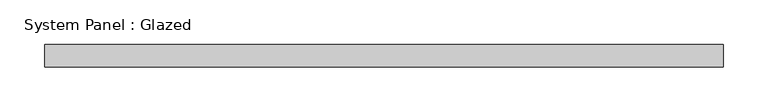
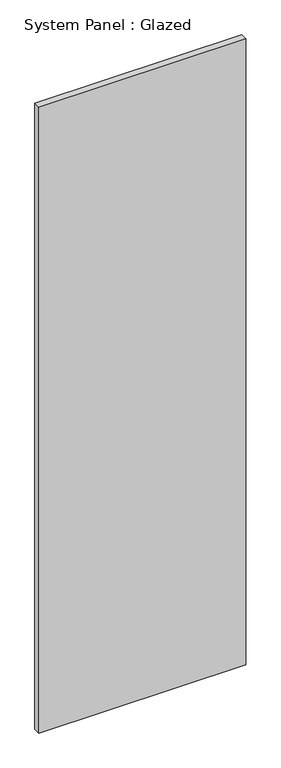
"""IFC4 building model written with IfcOpenShell, lengths in millimetres: plate geometry, System Panel : Glazed."""

from ifc_helpers import new_model, si_unit, origin, origin_with_axes, place, context, project, spatial, polyline, outline, extrude, source, transform, mapped, element, save


def system_panel_glazed_7cdb8ab2(model_context):
    return source(origin(), model_context, "Body", "SweptSolid", [
        extrude(outline(polyline([(381.0, 19.05), (-381.0, 19.05), (-381.0, 44.45), (381.0, 44.45), (381.0, 19.05)])), origin_with_axes(), (0.0, 0.0, 1.0), 2438.4),
    ])


if __name__ == "__main__":
    model = new_model("IFC4")
    model_context = context("Model", 3, world=origin())
    ifc_project = project(units=[si_unit("LENGTHUNIT", "METRE", prefix="MILLI")], contexts=[model_context])
    site = spatial("IfcSite", under=ifc_project)
    building = spatial("IfcBuilding", under=site)
    placement = place(None, origin())
    system_panel_glazed_shape = system_panel_glazed_7cdb8ab2(model_context)
    element("IfcPlate", 1, ObjectType="System Panel : Glazed", at=placement, inside=building, context=model_context, shape_type="MappedRepresentation", body=[
        mapped(system_panel_glazed_shape, transform((0.0, 0.0, 0.0), x_axis=(1.0, 0.0, 0.0), y_axis=(0.0, 1.0, 0.0), z_axis=(0.0, 0.0, 1.0))),
    ])
    save(model, "model.ifc")

# Revit data of these elements
# Type "System Panel : Glazed"
#   Construction Type Id = "GSP4R"
#   Analytic Construction = "1/8 in Pilkington single glazing"
#   Visual Light Transmittance = 0.9
#   Solar Heat Gain Coefficient = 0.86
#   Heat Transfer Coefficient (U) = 1.18115 BTU/(h·ft²·°F)
# Element 1 (IfcPlate, "System Panel : Glazed")
#   Materials on its faces: "Glass"
# Materials
#   "Glass": class "Glass", colour RGB 0 128 192, transparency 0.75, Description = "Soda Lime Glass", Cost = 0
